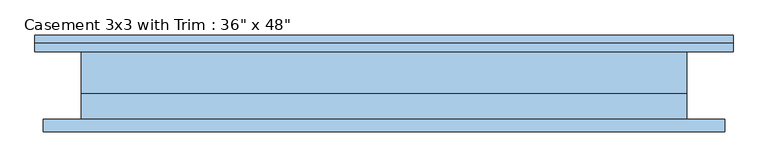
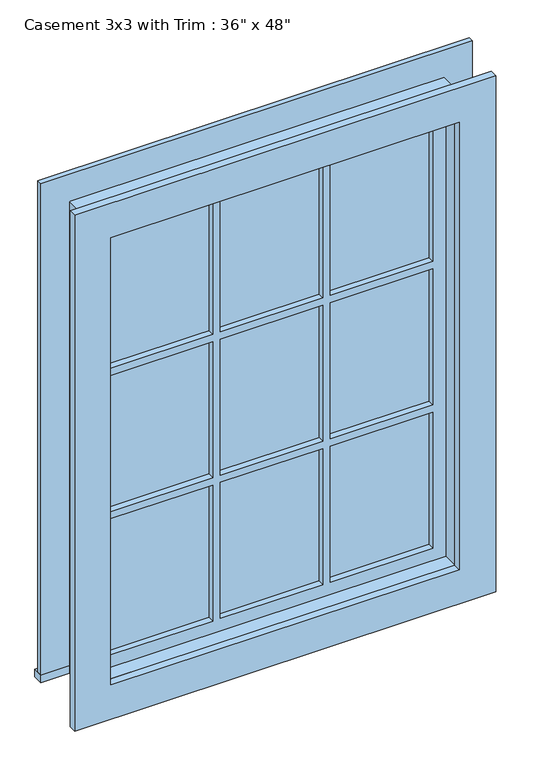
"""IFC4 building model written with IfcOpenShell, lengths in millimetres: window geometry."""

from ifc_helpers import new_model, si_unit, frame, origin, place, context, project, spatial, polyline, outline, extrude, source, transform, mapped, element, save


def window_ad8769eb(model_context):
    return source(origin(), model_context, "Body", "SweptSolid", [
        extrude(outline(polyline([(-527.05, 76.2), (527.05, 76.2), (527.05, 50.8), (-527.05, 50.8), (-527.05, 76.2)])), frame((0.0, 0.0, 914.4), z_axis=(0.0, 0.0, 1.0), x_axis=(1.0, 0.0, 0.0)), (0.0, 0.0, 1.0), 19.05),
        extrude(outline(polyline([(2114.55, -438.15), (2114.55, 438.15), (933.45, 438.15), (933.45, 527.05), (2203.45, 527.05), (2203.45, -527.05), (933.45, -527.05), (933.45, -438.15), (2114.55, -438.15)])), frame((0.0, 50.8, 0.0), z_axis=(0.0, 1.0, 0.0), x_axis=(0.0, 0.0, 1.0)), (0.0, 0.0, 1.0), 12.7),
        extrude(outline(polyline([(143.9333333, 15.875), (393.7, 15.875), (393.7, 3.175), (143.9333333, 3.175), (143.9333333, 15.875)])), frame((0.0, 0.0, 1718.7333333), z_axis=(0.0, 0.0, 1.0), x_axis=(1.0, 0.0, 0.0)), (0.0, 0.0, 1.0), 351.3666667),
        extrude(outline(polyline([(-124.8833333, 15.875), (124.8833333, 15.875), (124.8833333, 3.175), (-124.8833333, 3.175), (-124.8833333, 15.875)])), frame((0.0, 0.0, 1718.7333333), z_axis=(0.0, 0.0, 1.0), x_axis=(1.0, 0.0, 0.0)), (0.0, 0.0, 1.0), 351.3666667),
        extrude(outline(polyline([(-393.7, 15.875), (-143.9333333, 15.875), (-143.9333333, 3.175), (-393.7, 3.175), (-393.7, 15.875)])), frame((0.0, 0.0, 1718.7333333), z_axis=(0.0, 0.0, 1.0), x_axis=(1.0, 0.0, 0.0)), (0.0, 0.0, 1.0), 351.3666667),
        extrude(outline(polyline([(-393.7, 15.875), (-143.9333333, 15.875), (-143.9333333, 3.175), (-393.7, 3.175), (-393.7, 15.875)])), frame((0.0, 0.0, 1348.3166667), z_axis=(0.0, 0.0, 1.0), x_axis=(1.0, 0.0, 0.0)), (0.0, 0.0, 1.0), 351.3666667),
        extrude(outline(polyline([(-124.8833333, 15.875), (124.8833333, 15.875), (124.8833333, 3.175), (-124.8833333, 3.175), (-124.8833333, 15.875)])), frame((0.0, 0.0, 1348.3166667), z_axis=(0.0, 0.0, 1.0), x_axis=(1.0, 0.0, 0.0)), (0.0, 0.0, 1.0), 351.3666667),
        extrude(outline(polyline([(143.9333333, 15.875), (393.7, 15.875), (393.7, 3.175), (143.9333333, 3.175), (143.9333333, 15.875)])), frame((0.0, 0.0, 1348.3166667), z_axis=(0.0, 0.0, 1.0), x_axis=(1.0, 0.0, 0.0)), (0.0, 0.0, 1.0), 351.3666667),
        extrude(outline(polyline([(143.9333333, 15.875), (393.7, 15.875), (393.7, 3.175), (143.9333333, 3.175), (143.9333333, 15.875)])), frame((0.0, 0.0, 977.9), z_axis=(0.0, 0.0, 1.0), x_axis=(1.0, 0.0, 0.0)), (0.0, 0.0, 1.0), 351.3666667),
        extrude(outline(polyline([(-124.8833333, 15.875), (124.8833333, 15.875), (124.8833333, 3.175), (-124.8833333, 3.175), (-124.8833333, 15.875)])), frame((0.0, 0.0, 977.9), z_axis=(0.0, 0.0, 1.0), x_axis=(1.0, 0.0, 0.0)), (0.0, 0.0, 1.0), 351.3666667),
        extrude(outline(polyline([(-393.7, 15.875), (-143.9333333, 15.875), (-143.9333333, 3.175), (-393.7, 3.175), (-393.7, 15.875)])), frame((0.0, 0.0, 977.9), z_axis=(0.0, 0.0, 1.0), x_axis=(1.0, 0.0, 0.0)), (0.0, 0.0, 1.0), 351.3666667),
        extrude(outline(polyline([(2190.75, 514.35), (2190.75, -514.35), (857.25, -514.35), (857.25, 514.35), (2190.75, 514.35)]), holes=[polyline([(2101.85, 425.45), (946.15, 425.45), (946.15, -425.45), (2101.85, -425.45), (2101.85, 425.45)])]), frame((0.0, -69.85, 0.0), z_axis=(0.0, 1.0, 0.0), x_axis=(0.0, 0.0, 1.0)), (0.0, 0.0, 1.0), 19.05),
        extrude(outline(polyline([(2114.55, -438.15), (933.45, -438.15), (933.45, 438.15), (2114.55, 438.15), (2114.55, -438.15)]), holes=[polyline([(2070.1, -143.9333333), (1718.7333333, -143.9333333), (1718.7333333, -393.7), (2070.1, -393.7), (2070.1, -143.9333333)]), polyline([(1699.6833333, -143.9333333), (1348.3166667, -143.9333333), (1348.3166667, -393.7), (1699.6833333, -393.7), (1699.6833333, -143.9333333)]), polyline([(1329.2666667, -143.9333333), (977.9, -143.9333333), (977.9, -393.7), (1329.2666667, -393.7), (1329.2666667, -143.9333333)]), polyline([(2070.1, 124.8833333), (1718.7333333, 124.8833333), (1718.7333333, -124.8833333), (2070.1, -124.8833333), (2070.1, 124.8833333)]), polyline([(1699.6833333, 124.8833333), (1348.3166667, 124.8833333), (1348.3166667, -124.8833333), (1699.6833333, -124.8833333), (1699.6833333, 124.8833333)]), polyline([(1329.2666667, 124.8833333), (977.9, 124.8833333), (977.9, -124.8833333), (1329.2666667, -124.8833333), (1329.2666667, 124.8833333)]), polyline([(2070.1, 393.7), (1718.7333333, 393.7), (1718.7333333, 143.9333333), (2070.1, 143.9333333), (2070.1, 393.7)]), polyline([(1699.6833333, 393.7), (1348.3166667, 393.7), (1348.3166667, 143.9333333), (1699.6833333, 143.9333333), (1699.6833333, 393.7)]), polyline([(1329.2666667, 393.7), (977.9, 393.7), (977.9, 143.9333333), (1329.2666667, 143.9333333), (1329.2666667, 393.7)])]), frame((0.0, -12.7, 0.0), z_axis=(0.0, 1.0, 0.0), x_axis=(0.0, 0.0, 1.0)), (0.0, 0.0, 1.0), 44.45),
        extrude(outline(polyline([(2133.6, -457.2), (914.4, -457.2), (914.4, 457.2), (2133.6, 457.2), (2133.6, -457.2)]), holes=[polyline([(2101.85, -425.45), (2101.85, 425.45), (946.15, 425.45), (946.15, -425.45), (2101.85, -425.45)])]), frame((0.0, -50.8, 0.0), z_axis=(0.0, 1.0, 0.0), x_axis=(0.0, 0.0, 1.0)), (0.0, 0.0, 1.0), 38.1),
        extrude(outline(polyline([(2133.6, 457.2), (2133.6, -457.2), (914.4, -457.2), (914.4, 457.2), (2133.6, 457.2)]), holes=[polyline([(2114.55, 438.15), (933.45, 438.15), (933.45, -438.15), (2114.55, -438.15), (2114.55, 438.15)])]), frame((0.0, -12.7, 0.0), z_axis=(0.0, 1.0, 0.0), x_axis=(0.0, 0.0, 1.0)), (0.0, 0.0, 1.0), 63.5),
    ])


if __name__ == "__main__":
    model = new_model("IFC4")
    model_context = context("Model", 3, world=origin())
    ifc_project = project(units=[si_unit("LENGTHUNIT", "METRE", prefix="MILLI")], contexts=[model_context])
    site = spatial("IfcSite", under=ifc_project)
    building = spatial("IfcBuilding", under=site)
    placement = place(None, origin())
    window_shape = window_ad8769eb(model_context)
    element("IfcWindow", 1, ObjectType="Casement 3x3 with Trim : 36\" x 48\"", at=placement, inside=building, context=model_context, shape_type="MappedRepresentation", body=[
        mapped(window_shape, transform((0.0, 0.0, 0.0), x_axis=(1.0, 0.0, 0.0), y_axis=(0.0, 1.0, 0.0), z_axis=(0.0, 0.0, 1.0))),
    ])
    save(model, "model.ifc")

# Revit data of these elements
# Type "Casement 3x3 with Trim : 36\" x 48\""
#   Type Mark = "10"
#   Construction Type Id = "GSP4R"
#   Assembly Code = "B2020100"
#   Analytic Construction = "1/8 in Pilkington single glazing"
#   Visual Light Transmittance = 0.9
#   Solar Heat Gain Coefficient = 0.78
#   Heat Transfer Coefficient (U) = 0.6496 BTU/(h·ft²·°F)
#   Height = 4' - 0"
#   Default Sill Height = 3' - 0"
#   Trim Projection - Ext. = 0' - 0 1/2"
#   Trim Projection - Int. = 0' - 0 3/4"
#   Trim Width - Exterior = 0' - 3 1/2"
#   Trim Width - Interior = 0' - 3 1/2"
#   Width = 3' - 0"
#   Window Inset = 0' - 0 3/4"
#   Define Thermal Properties by = 1
#   Glass Pane Material = Glass
#   Sash Material = Sash
#   Trim Exterior Material = Trim
#   Trim Interior Material = Trim
#   Wall Closure = (empty or 0)
# Element 1 (IfcWindow, "Casement 3x3 with Trim : 36\" x 48\"")
#   Materials on its faces: "Sash", "Glass", "Trim"
# Materials
#   "Glass": class "Glass", colour RGB 0 128 192, transparency 0.75, Description = "Soda Lime Glass", Cost = 0
#   "Sash": class "Wood", colour RGB 224 178 126, transparency 0
#   "Trim": class "Wood", colour RGB 224 178 126, transparency 0
